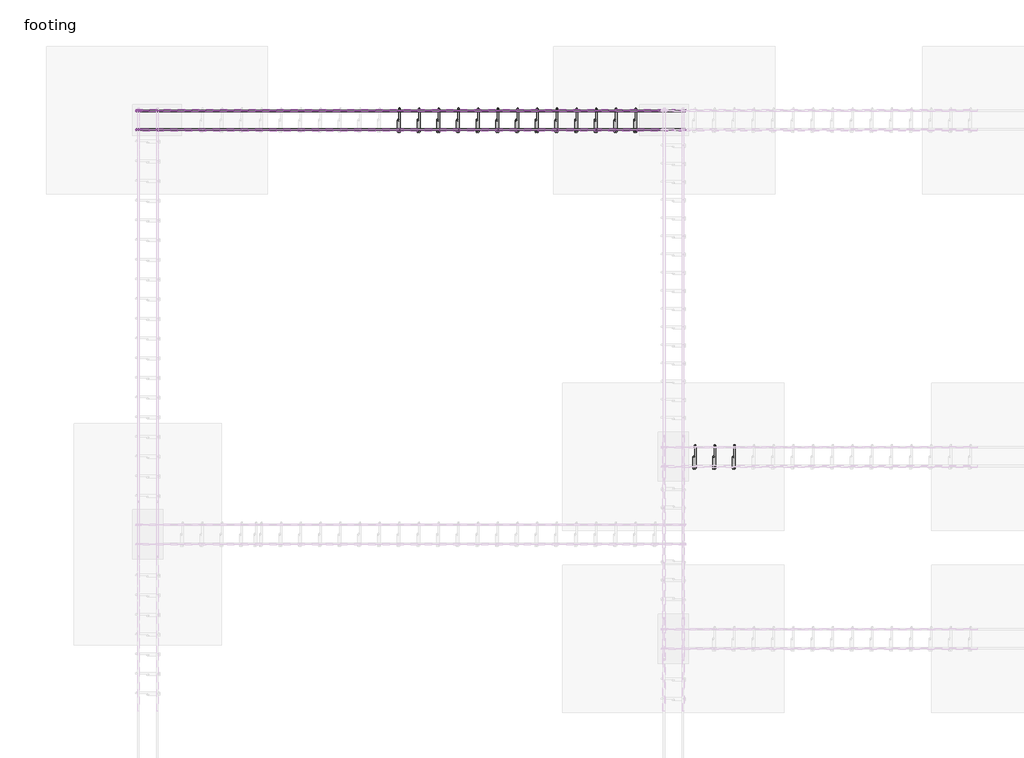
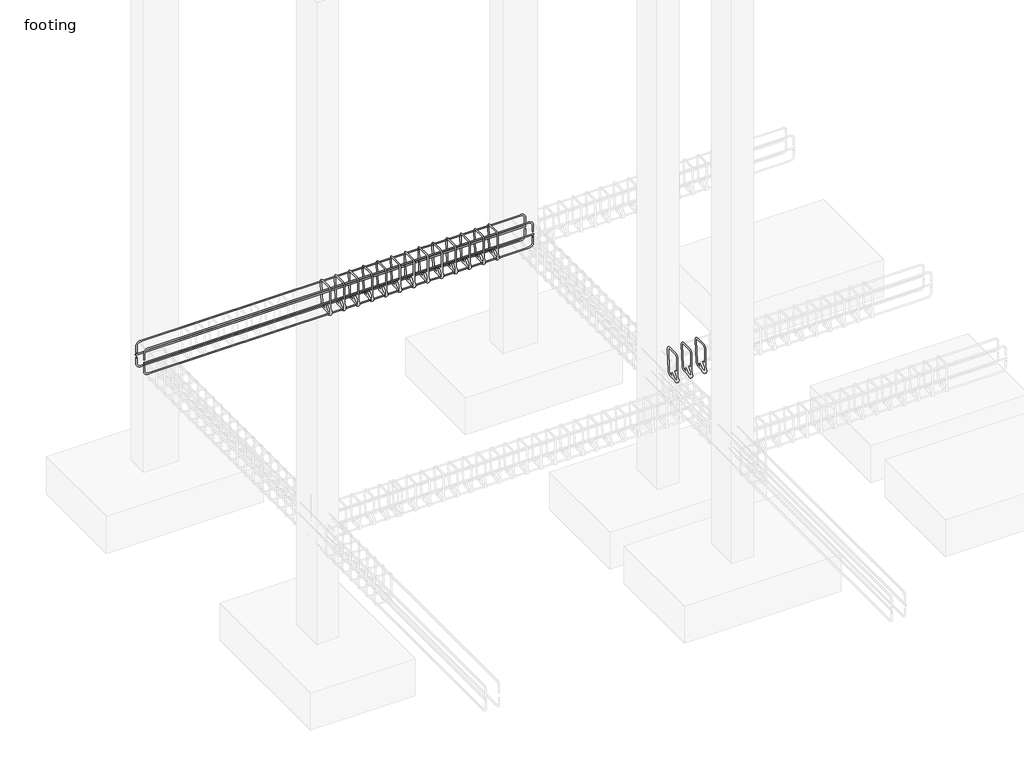
# One storey, part 17 of 21: 22 reinforcing bars.
"""IFC4 building model written with IfcOpenShell, lengths in millimetres."""

from ifc_helpers import new_model, si_unit, point, frame, origin, place, context, project, spatial, polyline, circle_curve, trimmed, segment, composite_curve, element, save
from ifc_brep_helpers import swept_disk

model = new_model("IFC4")

# Units and contexts
model_context = context("Model", 3, world=origin())
ifc_project = project(units=[si_unit("LENGTHUNIT", "METRE", prefix="MILLI")], contexts=[model_context])

# Site, building, storey
site = spatial("IfcSite", under=ifc_project)
building = spatial("IfcBuilding", under=site)
storey = spatial("IfcBuildingStorey", under=building, Name="footing", Elevation=-1524.0)

# Reinforcing bars
placement = place(None, origin())
element("IfcReinforcingBar", 1, at=placement, inside=storey, context=model_context, shape_type="SolidModel", body=[
    swept_disk(composite_curve([segment(polyline([(-7699.7883428, 8213.6387132, -310.8825168), (-7699.7883428, 8158.7737147, -365.7475153)]), True, "CONTINUOUS"), segment(trimmed(circle_curve(frame((-7699.7883428, 8136.3230744, -343.296875), z_axis=(-1.0, 0.0, 0.0), x_axis=(0.0, 22.450640299999577, -22.450640299999975)), 31.75), [point((-7699.7883428, 8158.7737147, -365.7475153))], [point((-7699.7883428, 8104.5730744, -343.296875))], True, "CARTESIAN"), True, "CONTINUOUS"), segment(polyline([(-7699.7883428, 8104.5730744, -343.296875), (-7699.7883428, 8104.5730744, -63.103125)]), True, "CONTINUOUS"), segment(trimmed(circle_curve(frame((-7699.7883428, 8136.3230744, -63.103125), z_axis=(-1.0, 0.0, 0.0), x_axis=(0.0, -31.75, 0.0)), 31.75), [point((-7699.7883428, 8104.5730744, -63.103125))], [point((-7699.7883428, 8136.3230744, -31.353125))], True, "CARTESIAN"), True, "CONTINUOUS"), segment(polyline([(-7699.7883428, 8136.3230744, -31.353125), (-7699.7883428, 8264.1168244, -31.353125)]), True, "CONTINUOUS"), segment(trimmed(circle_curve(frame((-7698.6159328, 8264.1168244, -63.0814712), z_axis=(-0.9993179916193466, 0.0, -0.03692629992126919), x_axis=(-1.1724099999992177, 0.0, 31.728346200000004)), 31.75), [point((-7699.7883428, 8264.1168244, -31.353125))], [point((-7698.6159328, 8295.8668244, -63.0814712))], True, "CARTESIAN"), True, "CONTINUOUS"), segment(polyline([(-7698.6159328, 8295.8668244, -63.0814712), (-7688.2607528, 8295.8668244, -343.3185288)]), True, "CONTINUOUS"), segment(trimmed(circle_curve(frame((-7688.2607528, 8264.1168244, -343.3185288), z_axis=(-0.9993179916193466, 0.0, -0.03692629992126919), x_axis=(0.0, 31.75, 0.0)), 31.75), [point((-7688.2607528, 8295.8668244, -343.3185288))], [point((-7687.0883428, 8264.1168244, -375.046875))], True, "CARTESIAN"), True, "CONTINUOUS"), segment(polyline([(-7687.0883428, 8264.1168244, -375.046875), (-7687.0883428, 8136.3230744, -375.046875)]), True, "CONTINUOUS"), segment(trimmed(circle_curve(frame((-7687.0883428, 8136.3230744, -343.296875), z_axis=(-1.0, 0.0, 0.0), x_axis=(0.0, 0.0, -31.75)), 31.75), [point((-7687.0883428, 8136.3230744, -375.046875))], [point((-7687.0883428, 8113.8724341, -320.8462347))], True, "CARTESIAN"), True, "CONTINUOUS"), segment(polyline([(-7687.0883428, 8113.8724341, -320.8462347), (-7687.0883428, 8168.7374326, -265.9812362)]), True, "CONTINUOUS")], self_intersect=False), 6.35),
])
element("IfcReinforcingBar", 2, at=placement, inside=storey, context=model_context, shape_type="SolidModel", body=[
    swept_disk(composite_curve([segment(polyline([(-7537.0883428, 8213.6387132, -310.8825168), (-7537.0883428, 8158.7737147, -365.7475153)]), True, "CONTINUOUS"), segment(trimmed(circle_curve(frame((-7537.0883428, 8136.3230744, -343.296875), z_axis=(-1.0, 0.0, 0.0), x_axis=(0.0, 22.450640299999577, -22.450640299999975)), 31.75), [point((-7537.0883428, 8158.7737147, -365.7475153))], [point((-7537.0883428, 8104.5730744, -343.296875))], True, "CARTESIAN"), True, "CONTINUOUS"), segment(polyline([(-7537.0883428, 8104.5730744, -343.296875), (-7537.0883428, 8104.5730744, -63.103125)]), True, "CONTINUOUS"), segment(trimmed(circle_curve(frame((-7537.0883428, 8136.3230744, -63.103125), z_axis=(-1.0, 0.0, 0.0), x_axis=(0.0, -31.75, 0.0)), 31.75), [point((-7537.0883428, 8104.5730744, -63.103125))], [point((-7537.0883428, 8136.3230744, -31.353125))], True, "CARTESIAN"), True, "CONTINUOUS"), segment(polyline([(-7537.0883428, 8136.3230744, -31.353125), (-7537.0883428, 8264.1168244, -31.353125)]), True, "CONTINUOUS"), segment(trimmed(circle_curve(frame((-7535.9159328, 8264.1168244, -63.0814712), z_axis=(-0.9993179916193466, 0.0, -0.03692629992126919), x_axis=(-1.1724100000001272, 0.0, 31.728346200000004)), 31.75), [point((-7537.0883428, 8264.1168244, -31.353125))], [point((-7535.9159328, 8295.8668244, -63.0814712))], True, "CARTESIAN"), True, "CONTINUOUS"), segment(polyline([(-7535.9159328, 8295.8668244, -63.0814712), (-7525.5607528, 8295.8668244, -343.3185288)]), True, "CONTINUOUS"), segment(trimmed(circle_curve(frame((-7525.5607528, 8264.1168244, -343.3185288), z_axis=(-0.9993179916193466, 0.0, -0.03692629992126919), x_axis=(0.0, 31.75, 0.0)), 31.75), [point((-7525.5607528, 8295.8668244, -343.3185288))], [point((-7524.3883428, 8264.1168244, -375.046875))], True, "CARTESIAN"), True, "CONTINUOUS"), segment(polyline([(-7524.3883428, 8264.1168244, -375.046875), (-7524.3883428, 8136.3230744, -375.046875)]), True, "CONTINUOUS"), segment(trimmed(circle_curve(frame((-7524.3883428, 8136.3230744, -343.296875), z_axis=(-1.0, 0.0, 0.0), x_axis=(0.0, 0.0, -31.75)), 31.75), [point((-7524.3883428, 8136.3230744, -375.046875))], [point((-7524.3883428, 8113.8724341, -320.8462347))], True, "CARTESIAN"), True, "CONTINUOUS"), segment(polyline([(-7524.3883428, 8113.8724341, -320.8462347), (-7524.3883428, 8168.7374326, -265.9812362)]), True, "CONTINUOUS")], self_intersect=False), 6.35),
])
element("IfcReinforcingBar", 3, at=placement, inside=storey, context=model_context, shape_type="SolidModel", body=[
    swept_disk(composite_curve([segment(polyline([(-7374.3883428, 8213.6387132, -310.8825168), (-7374.3883428, 8158.7737147, -365.7475153)]), True, "CONTINUOUS"), segment(trimmed(circle_curve(frame((-7374.3883428, 8136.3230744, -343.296875), z_axis=(-1.0, 0.0, 0.0), x_axis=(0.0, 22.450640299999577, -22.450640299999975)), 31.75), [point((-7374.3883428, 8158.7737147, -365.7475153))], [point((-7374.3883428, 8104.5730744, -343.296875))], True, "CARTESIAN"), True, "CONTINUOUS"), segment(polyline([(-7374.3883428, 8104.5730744, -343.296875), (-7374.3883428, 8104.5730744, -63.103125)]), True, "CONTINUOUS"), segment(trimmed(circle_curve(frame((-7374.3883428, 8136.3230744, -63.103125), z_axis=(-1.0, 0.0, 0.0), x_axis=(0.0, -31.75, 0.0)), 31.75), [point((-7374.3883428, 8104.5730744, -63.103125))], [point((-7374.3883428, 8136.3230744, -31.353125))], True, "CARTESIAN"), True, "CONTINUOUS"), segment(polyline([(-7374.3883428, 8136.3230744, -31.353125), (-7374.3883428, 8264.1168244, -31.353125)]), True, "CONTINUOUS"), segment(trimmed(circle_curve(frame((-7373.2159328, 8264.1168244, -63.0814712), z_axis=(-0.9993179916193466, 0.0, -0.03692629992126919), x_axis=(-1.1724100000001272, 0.0, 31.728346200000004)), 31.75), [point((-7374.3883428, 8264.1168244, -31.353125))], [point((-7373.2159328, 8295.8668244, -63.0814712))], True, "CARTESIAN"), True, "CONTINUOUS"), segment(polyline([(-7373.2159328, 8295.8668244, -63.0814712), (-7362.8607528, 8295.8668244, -343.3185288)]), True, "CONTINUOUS"), segment(trimmed(circle_curve(frame((-7362.8607528, 8264.1168244, -343.3185288), z_axis=(-0.9993179916193466, 0.0, -0.03692629992126919), x_axis=(0.0, 31.75, 0.0)), 31.75), [point((-7362.8607528, 8295.8668244, -343.3185288))], [point((-7361.6883428, 8264.1168244, -375.046875))], True, "CARTESIAN"), True, "CONTINUOUS"), segment(polyline([(-7361.6883428, 8264.1168244, -375.046875), (-7361.6883428, 8136.3230744, -375.046875)]), True, "CONTINUOUS"), segment(trimmed(circle_curve(frame((-7361.6883428, 8136.3230744, -343.296875), z_axis=(-1.0, 0.0, 0.0), x_axis=(0.0, 0.0, -31.75)), 31.75), [point((-7361.6883428, 8136.3230744, -375.046875))], [point((-7361.6883428, 8113.8724341, -320.8462347))], True, "CARTESIAN"), True, "CONTINUOUS"), segment(polyline([(-7361.6883428, 8113.8724341, -320.8462347), (-7361.6883428, 8168.7374326, -265.9812362)]), True, "CONTINUOUS")], self_intersect=False), 6.35),
])
element("IfcReinforcingBar", 4, at=placement, inside=storey, context=model_context, shape_type="SolidModel", body=[
    swept_disk(composite_curve([segment(polyline([(-10142.5883428, 10994.9387132, -310.8825168), (-10142.5883428, 10940.0737147, -365.7475153)]), True, "CONTINUOUS"), segment(trimmed(circle_curve(frame((-10142.5883428, 10917.6230744, -343.296875), z_axis=(-1.0, 0.0, 0.0), x_axis=(0.0, 22.450640299999577, -22.450640299999975)), 31.75), [point((-10142.5883428, 10940.0737147, -365.7475153))], [point((-10142.5883428, 10885.8730744, -343.296875))], True, "CARTESIAN"), True, "CONTINUOUS"), segment(polyline([(-10142.5883428, 10885.8730744, -343.296875), (-10142.5883428, 10885.8730744, -63.103125)]), True, "CONTINUOUS"), segment(trimmed(circle_curve(frame((-10142.5883428, 10917.6230744, -63.103125), z_axis=(-1.0, 0.0, 0.0), x_axis=(0.0, -31.75, 0.0)), 31.75), [point((-10142.5883428, 10885.8730744, -63.103125))], [point((-10142.5883428, 10917.6230744, -31.353125))], True, "CARTESIAN"), True, "CONTINUOUS"), segment(polyline([(-10142.5883428, 10917.6230744, -31.353125), (-10142.5883428, 11045.4168244, -31.353125)]), True, "CONTINUOUS"), segment(trimmed(circle_curve(frame((-10141.4159328, 11045.4168244, -63.0814712), z_axis=(-0.9993179916193466, 0.0, -0.03692629992126919), x_axis=(-1.1724099999992177, 0.0, 31.728346200000004)), 31.75), [point((-10142.5883428, 11045.4168244, -31.353125))], [point((-10141.4159328, 11077.1668244, -63.0814712))], True, "CARTESIAN"), True, "CONTINUOUS"), segment(polyline([(-10141.4159328, 11077.1668244, -63.0814712), (-10131.0607528, 11077.1668244, -343.3185288)]), True, "CONTINUOUS"), segment(trimmed(circle_curve(frame((-10131.0607528, 11045.4168244, -343.3185288), z_axis=(-0.9993179916193466, 0.0, -0.03692629992126919), x_axis=(0.0, 31.75, 0.0)), 31.75), [point((-10131.0607528, 11077.1668244, -343.3185288))], [point((-10129.8883428, 11045.4168244, -375.046875))], True, "CARTESIAN"), True, "CONTINUOUS"), segment(polyline([(-10129.8883428, 11045.4168244, -375.046875), (-10129.8883428, 10917.6230744, -375.046875)]), True, "CONTINUOUS"), segment(trimmed(circle_curve(frame((-10129.8883428, 10917.6230744, -343.296875), z_axis=(-1.0, 0.0, 0.0), x_axis=(0.0, 0.0, -31.75)), 31.75), [point((-10129.8883428, 10917.6230744, -375.046875))], [point((-10129.8883428, 10895.1724341, -320.8462347))], True, "CARTESIAN"), True, "CONTINUOUS"), segment(polyline([(-10129.8883428, 10895.1724341, -320.8462347), (-10129.8883428, 10950.0374326, -265.9812362)]), True, "CONTINUOUS")], self_intersect=False), 6.35),
])
element("IfcReinforcingBar", 5, at=placement, inside=storey, context=model_context, shape_type="SolidModel", body=[
    swept_disk(composite_curve([segment(polyline([(-9979.8883428, 10994.9387132, -310.8825168), (-9979.8883428, 10940.0737147, -365.7475153)]), True, "CONTINUOUS"), segment(trimmed(circle_curve(frame((-9979.8883428, 10917.6230744, -343.296875), z_axis=(-1.0, 0.0, 0.0), x_axis=(0.0, 22.450640299999577, -22.450640299999975)), 31.75), [point((-9979.8883428, 10940.0737147, -365.7475153))], [point((-9979.8883428, 10885.8730744, -343.296875))], True, "CARTESIAN"), True, "CONTINUOUS"), segment(polyline([(-9979.8883428, 10885.8730744, -343.296875), (-9979.8883428, 10885.8730744, -63.103125)]), True, "CONTINUOUS"), segment(trimmed(circle_curve(frame((-9979.8883428, 10917.6230744, -63.103125), z_axis=(-1.0, 0.0, 0.0), x_axis=(0.0, -31.75, 0.0)), 31.75), [point((-9979.8883428, 10885.8730744, -63.103125))], [point((-9979.8883428, 10917.6230744, -31.353125))], True, "CARTESIAN"), True, "CONTINUOUS"), segment(polyline([(-9979.8883428, 10917.6230744, -31.353125), (-9979.8883428, 11045.4168244, -31.353125)]), True, "CONTINUOUS"), segment(trimmed(circle_curve(frame((-9978.7159328, 11045.4168244, -63.0814712), z_axis=(-0.9993179916193466, 0.0, -0.03692629992126919), x_axis=(-1.1724100000010367, 0.0, 31.728346200000004)), 31.75), [point((-9979.8883428, 11045.4168244, -31.353125))], [point((-9978.7159328, 11077.1668244, -63.0814712))], True, "CARTESIAN"), True, "CONTINUOUS"), segment(polyline([(-9978.7159328, 11077.1668244, -63.0814712), (-9968.3607528, 11077.1668244, -343.3185288)]), True, "CONTINUOUS"), segment(trimmed(circle_curve(frame((-9968.3607528, 11045.4168244, -343.3185288), z_axis=(-0.9993179916193466, 0.0, -0.03692629992126919), x_axis=(0.0, 31.75, 0.0)), 31.75), [point((-9968.3607528, 11077.1668244, -343.3185288))], [point((-9967.1883428, 11045.4168244, -375.046875))], True, "CARTESIAN"), True, "CONTINUOUS"), segment(polyline([(-9967.1883428, 11045.4168244, -375.046875), (-9967.1883428, 10917.6230744, -375.046875)]), True, "CONTINUOUS"), segment(trimmed(circle_curve(frame((-9967.1883428, 10917.6230744, -343.296875), z_axis=(-1.0, 0.0, 0.0), x_axis=(0.0, 0.0, -31.75)), 31.75), [point((-9967.1883428, 10917.6230744, -375.046875))], [point((-9967.1883428, 10895.1724341, -320.8462347))], True, "CARTESIAN"), True, "CONTINUOUS"), segment(polyline([(-9967.1883428, 10895.1724341, -320.8462347), (-9967.1883428, 10950.0374326, -265.9812362)]), True, "CONTINUOUS")], self_intersect=False), 6.35),
])
element("IfcReinforcingBar", 6, at=placement, inside=storey, context=model_context, shape_type="SolidModel", body=[
    swept_disk(composite_curve([segment(polyline([(-9817.1883428, 10994.9387132, -310.8825168), (-9817.1883428, 10940.0737147, -365.7475153)]), True, "CONTINUOUS"), segment(trimmed(circle_curve(frame((-9817.1883428, 10917.6230744, -343.296875), z_axis=(-1.0, 0.0, 0.0), x_axis=(0.0, 22.450640299999577, -22.450640299999975)), 31.75), [point((-9817.1883428, 10940.0737147, -365.7475153))], [point((-9817.1883428, 10885.8730744, -343.296875))], True, "CARTESIAN"), True, "CONTINUOUS"), segment(polyline([(-9817.1883428, 10885.8730744, -343.296875), (-9817.1883428, 10885.8730744, -63.103125)]), True, "CONTINUOUS"), segment(trimmed(circle_curve(frame((-9817.1883428, 10917.6230744, -63.103125), z_axis=(-1.0, 0.0, 0.0), x_axis=(0.0, -31.75, 0.0)), 31.75), [point((-9817.1883428, 10885.8730744, -63.103125))], [point((-9817.1883428, 10917.6230744, -31.353125))], True, "CARTESIAN"), True, "CONTINUOUS"), segment(polyline([(-9817.1883428, 10917.6230744, -31.353125), (-9817.1883428, 11045.4168244, -31.353125)]), True, "CONTINUOUS"), segment(trimmed(circle_curve(frame((-9816.0159328, 11045.4168244, -63.0814712), z_axis=(-0.9993179916193466, 0.0, -0.03692629992126919), x_axis=(-1.1724099999992177, 0.0, 31.728346200000004)), 31.75), [point((-9817.1883428, 11045.4168244, -31.353125))], [point((-9816.0159328, 11077.1668244, -63.0814712))], True, "CARTESIAN"), True, "CONTINUOUS"), segment(polyline([(-9816.0159328, 11077.1668244, -63.0814712), (-9805.6607528, 11077.1668244, -343.3185288)]), True, "CONTINUOUS"), segment(trimmed(circle_curve(frame((-9805.6607528, 11045.4168244, -343.3185288), z_axis=(-0.9993179916193466, 0.0, -0.03692629992126919), x_axis=(0.0, 31.75, 0.0)), 31.75), [point((-9805.6607528, 11077.1668244, -343.3185288))], [point((-9804.4883428, 11045.4168244, -375.046875))], True, "CARTESIAN"), True, "CONTINUOUS"), segment(polyline([(-9804.4883428, 11045.4168244, -375.046875), (-9804.4883428, 10917.6230744, -375.046875)]), True, "CONTINUOUS"), segment(trimmed(circle_curve(frame((-9804.4883428, 10917.6230744, -343.296875), z_axis=(-1.0, 0.0, 0.0), x_axis=(0.0, 0.0, -31.75)), 31.75), [point((-9804.4883428, 10917.6230744, -375.046875))], [point((-9804.4883428, 10895.1724341, -320.8462347))], True, "CARTESIAN"), True, "CONTINUOUS"), segment(polyline([(-9804.4883428, 10895.1724341, -320.8462347), (-9804.4883428, 10950.0374326, -265.9812362)]), True, "CONTINUOUS")], self_intersect=False), 6.35),
])
element("IfcReinforcingBar", 7, at=placement, inside=storey, context=model_context, shape_type="SolidModel", body=[
    swept_disk(composite_curve([segment(polyline([(-9654.4883428, 10994.9387132, -310.8825168), (-9654.4883428, 10940.0737147, -365.7475153)]), True, "CONTINUOUS"), segment(trimmed(circle_curve(frame((-9654.4883428, 10917.6230744, -343.296875), z_axis=(-1.0, 0.0, 0.0), x_axis=(0.0, 22.450640299999577, -22.450640299999975)), 31.75), [point((-9654.4883428, 10940.0737147, -365.7475153))], [point((-9654.4883428, 10885.8730744, -343.296875))], True, "CARTESIAN"), True, "CONTINUOUS"), segment(polyline([(-9654.4883428, 10885.8730744, -343.296875), (-9654.4883428, 10885.8730744, -63.103125)]), True, "CONTINUOUS"), segment(trimmed(circle_curve(frame((-9654.4883428, 10917.6230744, -63.103125), z_axis=(-1.0, 0.0, 0.0), x_axis=(0.0, -31.75, 0.0)), 31.75), [point((-9654.4883428, 10885.8730744, -63.103125))], [point((-9654.4883428, 10917.6230744, -31.353125))], True, "CARTESIAN"), True, "CONTINUOUS"), segment(polyline([(-9654.4883428, 10917.6230744, -31.353125), (-9654.4883428, 11045.4168244, -31.353125)]), True, "CONTINUOUS"), segment(trimmed(circle_curve(frame((-9653.3159328, 11045.4168244, -63.0814712), z_axis=(-0.9993179916193466, 0.0, -0.03692629992126919), x_axis=(-1.1724099999992177, 0.0, 31.728346200000004)), 31.75), [point((-9654.4883428, 11045.4168244, -31.353125))], [point((-9653.3159328, 11077.1668244, -63.0814712))], True, "CARTESIAN"), True, "CONTINUOUS"), segment(polyline([(-9653.3159328, 11077.1668244, -63.0814712), (-9642.9607528, 11077.1668244, -343.3185288)]), True, "CONTINUOUS"), segment(trimmed(circle_curve(frame((-9642.9607528, 11045.4168244, -343.3185288), z_axis=(-0.9993179916193466, 0.0, -0.03692629992126919), x_axis=(0.0, 31.75, 0.0)), 31.75), [point((-9642.9607528, 11077.1668244, -343.3185288))], [point((-9641.7883428, 11045.4168244, -375.046875))], True, "CARTESIAN"), True, "CONTINUOUS"), segment(polyline([(-9641.7883428, 11045.4168244, -375.046875), (-9641.7883428, 10917.6230744, -375.046875)]), True, "CONTINUOUS"), segment(trimmed(circle_curve(frame((-9641.7883428, 10917.6230744, -343.296875), z_axis=(-1.0, 0.0, 0.0), x_axis=(0.0, 0.0, -31.75)), 31.75), [point((-9641.7883428, 10917.6230744, -375.046875))], [point((-9641.7883428, 10895.1724341, -320.8462347))], True, "CARTESIAN"), True, "CONTINUOUS"), segment(polyline([(-9641.7883428, 10895.1724341, -320.8462347), (-9641.7883428, 10950.0374326, -265.9812362)]), True, "CONTINUOUS")], self_intersect=False), 6.35),
])
element("IfcReinforcingBar", 8, at=placement, inside=storey, context=model_context, shape_type="SolidModel", body=[
    swept_disk(composite_curve([segment(polyline([(-9491.7883428, 10994.9387132, -310.8825168), (-9491.7883428, 10940.0737147, -365.7475153)]), True, "CONTINUOUS"), segment(trimmed(circle_curve(frame((-9491.7883428, 10917.6230744, -343.296875), z_axis=(-1.0, 0.0, 0.0), x_axis=(0.0, 22.450640299999577, -22.450640299999975)), 31.75), [point((-9491.7883428, 10940.0737147, -365.7475153))], [point((-9491.7883428, 10885.8730744, -343.296875))], True, "CARTESIAN"), True, "CONTINUOUS"), segment(polyline([(-9491.7883428, 10885.8730744, -343.296875), (-9491.7883428, 10885.8730744, -63.103125)]), True, "CONTINUOUS"), segment(trimmed(circle_curve(frame((-9491.7883428, 10917.6230744, -63.103125), z_axis=(-1.0, 0.0, 0.0), x_axis=(0.0, -31.75, 0.0)), 31.75), [point((-9491.7883428, 10885.8730744, -63.103125))], [point((-9491.7883428, 10917.6230744, -31.353125))], True, "CARTESIAN"), True, "CONTINUOUS"), segment(polyline([(-9491.7883428, 10917.6230744, -31.353125), (-9491.7883428, 11045.4168244, -31.353125)]), True, "CONTINUOUS"), segment(trimmed(circle_curve(frame((-9490.6159328, 11045.4168244, -63.0814712), z_axis=(-0.9993179916193466, 0.0, -0.03692629992126919), x_axis=(-1.1724100000010367, 0.0, 31.728346200000004)), 31.75), [point((-9491.7883428, 11045.4168244, -31.353125))], [point((-9490.6159328, 11077.1668244, -63.0814712))], True, "CARTESIAN"), True, "CONTINUOUS"), segment(polyline([(-9490.6159328, 11077.1668244, -63.0814712), (-9480.2607528, 11077.1668244, -343.3185288)]), True, "CONTINUOUS"), segment(trimmed(circle_curve(frame((-9480.2607528, 11045.4168244, -343.3185288), z_axis=(-0.9993179916193466, 0.0, -0.03692629992126919), x_axis=(0.0, 31.75, 0.0)), 31.75), [point((-9480.2607528, 11077.1668244, -343.3185288))], [point((-9479.0883428, 11045.4168244, -375.046875))], True, "CARTESIAN"), True, "CONTINUOUS"), segment(polyline([(-9479.0883428, 11045.4168244, -375.046875), (-9479.0883428, 10917.6230744, -375.046875)]), True, "CONTINUOUS"), segment(trimmed(circle_curve(frame((-9479.0883428, 10917.6230744, -343.296875), z_axis=(-1.0, 0.0, 0.0), x_axis=(0.0, 0.0, -31.75)), 31.75), [point((-9479.0883428, 10917.6230744, -375.046875))], [point((-9479.0883428, 10895.1724341, -320.8462347))], True, "CARTESIAN"), True, "CONTINUOUS"), segment(polyline([(-9479.0883428, 10895.1724341, -320.8462347), (-9479.0883428, 10950.0374326, -265.9812362)]), True, "CONTINUOUS")], self_intersect=False), 6.35),
])
element("IfcReinforcingBar", 9, at=placement, inside=storey, context=model_context, shape_type="SolidModel", body=[
    swept_disk(composite_curve([segment(polyline([(-9329.0883428, 10994.9387132, -310.8825168), (-9329.0883428, 10940.0737147, -365.7475153)]), True, "CONTINUOUS"), segment(trimmed(circle_curve(frame((-9329.0883428, 10917.6230744, -343.296875), z_axis=(-1.0, 0.0, 0.0), x_axis=(0.0, 22.450640299999577, -22.450640299999975)), 31.75), [point((-9329.0883428, 10940.0737147, -365.7475153))], [point((-9329.0883428, 10885.8730744, -343.296875))], True, "CARTESIAN"), True, "CONTINUOUS"), segment(polyline([(-9329.0883428, 10885.8730744, -343.296875), (-9329.0883428, 10885.8730744, -63.103125)]), True, "CONTINUOUS"), segment(trimmed(circle_curve(frame((-9329.0883428, 10917.6230744, -63.103125), z_axis=(-1.0, 0.0, 0.0), x_axis=(0.0, -31.75, 0.0)), 31.75), [point((-9329.0883428, 10885.8730744, -63.103125))], [point((-9329.0883428, 10917.6230744, -31.353125))], True, "CARTESIAN"), True, "CONTINUOUS"), segment(polyline([(-9329.0883428, 10917.6230744, -31.353125), (-9329.0883428, 11045.4168244, -31.353125)]), True, "CONTINUOUS"), segment(trimmed(circle_curve(frame((-9327.9159328, 11045.4168244, -63.0814712), z_axis=(-0.9993179916193466, 0.0, -0.03692629992126919), x_axis=(-1.1724099999992177, 0.0, 31.728346200000004)), 31.75), [point((-9329.0883428, 11045.4168244, -31.353125))], [point((-9327.9159328, 11077.1668244, -63.0814712))], True, "CARTESIAN"), True, "CONTINUOUS"), segment(polyline([(-9327.9159328, 11077.1668244, -63.0814712), (-9317.5607528, 11077.1668244, -343.3185288)]), True, "CONTINUOUS"), segment(trimmed(circle_curve(frame((-9317.5607528, 11045.4168244, -343.3185288), z_axis=(-0.9993179916193466, 0.0, -0.03692629992126919), x_axis=(0.0, 31.75, 0.0)), 31.75), [point((-9317.5607528, 11077.1668244, -343.3185288))], [point((-9316.3883428, 11045.4168244, -375.046875))], True, "CARTESIAN"), True, "CONTINUOUS"), segment(polyline([(-9316.3883428, 11045.4168244, -375.046875), (-9316.3883428, 10917.6230744, -375.046875)]), True, "CONTINUOUS"), segment(trimmed(circle_curve(frame((-9316.3883428, 10917.6230744, -343.296875), z_axis=(-1.0, 0.0, 0.0), x_axis=(0.0, 0.0, -31.75)), 31.75), [point((-9316.3883428, 10917.6230744, -375.046875))], [point((-9316.3883428, 10895.1724341, -320.8462347))], True, "CARTESIAN"), True, "CONTINUOUS"), segment(polyline([(-9316.3883428, 10895.1724341, -320.8462347), (-9316.3883428, 10950.0374326, -265.9812362)]), True, "CONTINUOUS")], self_intersect=False), 6.35),
])
element("IfcReinforcingBar", 10, at=placement, inside=storey, context=model_context, shape_type="SolidModel", body=[
    swept_disk(composite_curve([segment(polyline([(-9166.3883428, 10994.9387132, -310.8825168), (-9166.3883428, 10940.0737147, -365.7475153)]), True, "CONTINUOUS"), segment(trimmed(circle_curve(frame((-9166.3883428, 10917.6230744, -343.296875), z_axis=(-1.0, 0.0, 0.0), x_axis=(0.0, 22.450640299999577, -22.450640299999975)), 31.75), [point((-9166.3883428, 10940.0737147, -365.7475153))], [point((-9166.3883428, 10885.8730744, -343.296875))], True, "CARTESIAN"), True, "CONTINUOUS"), segment(polyline([(-9166.3883428, 10885.8730744, -343.296875), (-9166.3883428, 10885.8730744, -63.103125)]), True, "CONTINUOUS"), segment(trimmed(circle_curve(frame((-9166.3883428, 10917.6230744, -63.103125), z_axis=(-1.0, 0.0, 0.0), x_axis=(0.0, -31.75, 0.0)), 31.75), [point((-9166.3883428, 10885.8730744, -63.103125))], [point((-9166.3883428, 10917.6230744, -31.353125))], True, "CARTESIAN"), True, "CONTINUOUS"), segment(polyline([(-9166.3883428, 10917.6230744, -31.353125), (-9166.3883428, 11045.4168244, -31.353125)]), True, "CONTINUOUS"), segment(trimmed(circle_curve(frame((-9165.2159328, 11045.4168244, -63.0814712), z_axis=(-0.9993179916193466, 0.0, -0.03692629992126919), x_axis=(-1.1724100000010367, 0.0, 31.728346200000004)), 31.75), [point((-9166.3883428, 11045.4168244, -31.353125))], [point((-9165.2159328, 11077.1668244, -63.0814712))], True, "CARTESIAN"), True, "CONTINUOUS"), segment(polyline([(-9165.2159328, 11077.1668244, -63.0814712), (-9154.8607528, 11077.1668244, -343.3185288)]), True, "CONTINUOUS"), segment(trimmed(circle_curve(frame((-9154.8607528, 11045.4168244, -343.3185288), z_axis=(-0.9993179916193466, 0.0, -0.03692629992126919), x_axis=(0.0, 31.75, 0.0)), 31.75), [point((-9154.8607528, 11077.1668244, -343.3185288))], [point((-9153.6883428, 11045.4168244, -375.046875))], True, "CARTESIAN"), True, "CONTINUOUS"), segment(polyline([(-9153.6883428, 11045.4168244, -375.046875), (-9153.6883428, 10917.6230744, -375.046875)]), True, "CONTINUOUS"), segment(trimmed(circle_curve(frame((-9153.6883428, 10917.6230744, -343.296875), z_axis=(-1.0, 0.0, 0.0), x_axis=(0.0, 0.0, -31.75)), 31.75), [point((-9153.6883428, 10917.6230744, -375.046875))], [point((-9153.6883428, 10895.1724341, -320.8462347))], True, "CARTESIAN"), True, "CONTINUOUS"), segment(polyline([(-9153.6883428, 10895.1724341, -320.8462347), (-9153.6883428, 10950.0374326, -265.9812362)]), True, "CONTINUOUS")], self_intersect=False), 6.35),
])
element("IfcReinforcingBar", 11, at=placement, inside=storey, context=model_context, shape_type="SolidModel", body=[
    swept_disk(composite_curve([segment(polyline([(-9003.6883428, 10994.9387132, -310.8825168), (-9003.6883428, 10940.0737147, -365.7475153)]), True, "CONTINUOUS"), segment(trimmed(circle_curve(frame((-9003.6883428, 10917.6230744, -343.296875), z_axis=(-1.0, 0.0, 0.0), x_axis=(0.0, 22.450640299999577, -22.450640299999975)), 31.75), [point((-9003.6883428, 10940.0737147, -365.7475153))], [point((-9003.6883428, 10885.8730744, -343.296875))], True, "CARTESIAN"), True, "CONTINUOUS"), segment(polyline([(-9003.6883428, 10885.8730744, -343.296875), (-9003.6883428, 10885.8730744, -63.103125)]), True, "CONTINUOUS"), segment(trimmed(circle_curve(frame((-9003.6883428, 10917.6230744, -63.103125), z_axis=(-1.0, 0.0, 0.0), x_axis=(0.0, -31.75, 0.0)), 31.75), [point((-9003.6883428, 10885.8730744, -63.103125))], [point((-9003.6883428, 10917.6230744, -31.353125))], True, "CARTESIAN"), True, "CONTINUOUS"), segment(polyline([(-9003.6883428, 10917.6230744, -31.353125), (-9003.6883428, 11045.4168244, -31.353125)]), True, "CONTINUOUS"), segment(trimmed(circle_curve(frame((-9002.5159328, 11045.4168244, -63.0814712), z_axis=(-0.9993179916193466, 0.0, -0.03692629992126919), x_axis=(-1.1724099999992177, 0.0, 31.728346200000004)), 31.75), [point((-9003.6883428, 11045.4168244, -31.353125))], [point((-9002.5159328, 11077.1668244, -63.0814712))], True, "CARTESIAN"), True, "CONTINUOUS"), segment(polyline([(-9002.5159328, 11077.1668244, -63.0814712), (-8992.1607528, 11077.1668244, -343.3185288)]), True, "CONTINUOUS"), segment(trimmed(circle_curve(frame((-8992.1607528, 11045.4168244, -343.3185288), z_axis=(-0.9993179916193466, 0.0, -0.03692629992126919), x_axis=(0.0, 31.75, 0.0)), 31.75), [point((-8992.1607528, 11077.1668244, -343.3185288))], [point((-8990.9883428, 11045.4168244, -375.046875))], True, "CARTESIAN"), True, "CONTINUOUS"), segment(polyline([(-8990.9883428, 11045.4168244, -375.046875), (-8990.9883428, 10917.6230744, -375.046875)]), True, "CONTINUOUS"), segment(trimmed(circle_curve(frame((-8990.9883428, 10917.6230744, -343.296875), z_axis=(-1.0, 0.0, 0.0), x_axis=(0.0, 0.0, -31.75)), 31.75), [point((-8990.9883428, 10917.6230744, -375.046875))], [point((-8990.9883428, 10895.1724341, -320.8462347))], True, "CARTESIAN"), True, "CONTINUOUS"), segment(polyline([(-8990.9883428, 10895.1724341, -320.8462347), (-8990.9883428, 10950.0374326, -265.9812362)]), True, "CONTINUOUS")], self_intersect=False), 6.35),
])
element("IfcReinforcingBar", 12, at=placement, inside=storey, context=model_context, shape_type="SolidModel", body=[
    swept_disk(composite_curve([segment(polyline([(-8840.9883428, 10994.9387132, -310.8825168), (-8840.9883428, 10940.0737147, -365.7475153)]), True, "CONTINUOUS"), segment(trimmed(circle_curve(frame((-8840.9883428, 10917.6230744, -343.296875), z_axis=(-1.0, 0.0, 0.0), x_axis=(0.0, 22.450640299999577, -22.450640299999975)), 31.75), [point((-8840.9883428, 10940.0737147, -365.7475153))], [point((-8840.9883428, 10885.8730744, -343.296875))], True, "CARTESIAN"), True, "CONTINUOUS"), segment(polyline([(-8840.9883428, 10885.8730744, -343.296875), (-8840.9883428, 10885.8730744, -63.103125)]), True, "CONTINUOUS"), segment(trimmed(circle_curve(frame((-8840.9883428, 10917.6230744, -63.103125), z_axis=(-1.0, 0.0, 0.0), x_axis=(0.0, -31.75, 0.0)), 31.75), [point((-8840.9883428, 10885.8730744, -63.103125))], [point((-8840.9883428, 10917.6230744, -31.353125))], True, "CARTESIAN"), True, "CONTINUOUS"), segment(polyline([(-8840.9883428, 10917.6230744, -31.353125), (-8840.9883428, 11045.4168244, -31.353125)]), True, "CONTINUOUS"), segment(trimmed(circle_curve(frame((-8839.8159328, 11045.4168244, -63.0814712), z_axis=(-0.9993179916193466, 0.0, -0.03692629992126919), x_axis=(-1.1724099999992177, 0.0, 31.728346200000004)), 31.75), [point((-8840.9883428, 11045.4168244, -31.353125))], [point((-8839.8159328, 11077.1668244, -63.0814712))], True, "CARTESIAN"), True, "CONTINUOUS"), segment(polyline([(-8839.8159328, 11077.1668244, -63.0814712), (-8829.4607528, 11077.1668244, -343.3185288)]), True, "CONTINUOUS"), segment(trimmed(circle_curve(frame((-8829.4607528, 11045.4168244, -343.3185288), z_axis=(-0.9993179916193466, 0.0, -0.03692629992126919), x_axis=(0.0, 31.75, 0.0)), 31.75), [point((-8829.4607528, 11077.1668244, -343.3185288))], [point((-8828.2883428, 11045.4168244, -375.046875))], True, "CARTESIAN"), True, "CONTINUOUS"), segment(polyline([(-8828.2883428, 11045.4168244, -375.046875), (-8828.2883428, 10917.6230744, -375.046875)]), True, "CONTINUOUS"), segment(trimmed(circle_curve(frame((-8828.2883428, 10917.6230744, -343.296875), z_axis=(-1.0, 0.0, 0.0), x_axis=(0.0, 0.0, -31.75)), 31.75), [point((-8828.2883428, 10917.6230744, -375.046875))], [point((-8828.2883428, 10895.1724341, -320.8462347))], True, "CARTESIAN"), True, "CONTINUOUS"), segment(polyline([(-8828.2883428, 10895.1724341, -320.8462347), (-8828.2883428, 10950.0374326, -265.9812362)]), True, "CONTINUOUS")], self_intersect=False), 6.35),
])
element("IfcReinforcingBar", 13, at=placement, inside=storey, context=model_context, shape_type="SolidModel", body=[
    swept_disk(composite_curve([segment(polyline([(-8678.2883428, 10994.9387132, -310.8825168), (-8678.2883428, 10940.0737147, -365.7475153)]), True, "CONTINUOUS"), segment(trimmed(circle_curve(frame((-8678.2883428, 10917.6230744, -343.296875), z_axis=(-1.0, 0.0, 0.0), x_axis=(0.0, 22.450640299999577, -22.450640299999975)), 31.75), [point((-8678.2883428, 10940.0737147, -365.7475153))], [point((-8678.2883428, 10885.8730744, -343.296875))], True, "CARTESIAN"), True, "CONTINUOUS"), segment(polyline([(-8678.2883428, 10885.8730744, -343.296875), (-8678.2883428, 10885.8730744, -63.103125)]), True, "CONTINUOUS"), segment(trimmed(circle_curve(frame((-8678.2883428, 10917.6230744, -63.103125), z_axis=(-1.0, 0.0, 0.0), x_axis=(0.0, -31.75, 0.0)), 31.75), [point((-8678.2883428, 10885.8730744, -63.103125))], [point((-8678.2883428, 10917.6230744, -31.353125))], True, "CARTESIAN"), True, "CONTINUOUS"), segment(polyline([(-8678.2883428, 10917.6230744, -31.353125), (-8678.2883428, 11045.4168244, -31.353125)]), True, "CONTINUOUS"), segment(trimmed(circle_curve(frame((-8677.1159328, 11045.4168244, -63.0814712), z_axis=(-0.9993179916193466, 0.0, -0.03692629992126919), x_axis=(-1.1724100000010367, 0.0, 31.728346200000004)), 31.75), [point((-8678.2883428, 11045.4168244, -31.353125))], [point((-8677.1159328, 11077.1668244, -63.0814712))], True, "CARTESIAN"), True, "CONTINUOUS"), segment(polyline([(-8677.1159328, 11077.1668244, -63.0814712), (-8666.7607528, 11077.1668244, -343.3185288)]), True, "CONTINUOUS"), segment(trimmed(circle_curve(frame((-8666.7607528, 11045.4168244, -343.3185288), z_axis=(-0.9993179916193466, 0.0, -0.03692629992126919), x_axis=(0.0, 31.75, 0.0)), 31.75), [point((-8666.7607528, 11077.1668244, -343.3185288))], [point((-8665.5883428, 11045.4168244, -375.046875))], True, "CARTESIAN"), True, "CONTINUOUS"), segment(polyline([(-8665.5883428, 11045.4168244, -375.046875), (-8665.5883428, 10917.6230744, -375.046875)]), True, "CONTINUOUS"), segment(trimmed(circle_curve(frame((-8665.5883428, 10917.6230744, -343.296875), z_axis=(-1.0, 0.0, 0.0), x_axis=(0.0, 0.0, -31.75)), 31.75), [point((-8665.5883428, 10917.6230744, -375.046875))], [point((-8665.5883428, 10895.1724341, -320.8462347))], True, "CARTESIAN"), True, "CONTINUOUS"), segment(polyline([(-8665.5883428, 10895.1724341, -320.8462347), (-8665.5883428, 10950.0374326, -265.9812362)]), True, "CONTINUOUS")], self_intersect=False), 6.35),
])
element("IfcReinforcingBar", 14, at=placement, inside=storey, context=model_context, shape_type="SolidModel", body=[
    swept_disk(composite_curve([segment(polyline([(-8515.5883428, 10994.9387132, -310.8825168), (-8515.5883428, 10940.0737147, -365.7475153)]), True, "CONTINUOUS"), segment(trimmed(circle_curve(frame((-8515.5883428, 10917.6230744, -343.296875), z_axis=(-1.0, 0.0, 0.0), x_axis=(0.0, 22.450640299999577, -22.450640299999975)), 31.75), [point((-8515.5883428, 10940.0737147, -365.7475153))], [point((-8515.5883428, 10885.8730744, -343.296875))], True, "CARTESIAN"), True, "CONTINUOUS"), segment(polyline([(-8515.5883428, 10885.8730744, -343.296875), (-8515.5883428, 10885.8730744, -63.103125)]), True, "CONTINUOUS"), segment(trimmed(circle_curve(frame((-8515.5883428, 10917.6230744, -63.103125), z_axis=(-1.0, 0.0, 0.0), x_axis=(0.0, -31.75, 0.0)), 31.75), [point((-8515.5883428, 10885.8730744, -63.103125))], [point((-8515.5883428, 10917.6230744, -31.353125))], True, "CARTESIAN"), True, "CONTINUOUS"), segment(polyline([(-8515.5883428, 10917.6230744, -31.353125), (-8515.5883428, 11045.4168244, -31.353125)]), True, "CONTINUOUS"), segment(trimmed(circle_curve(frame((-8514.4159328, 11045.4168244, -63.0814712), z_axis=(-0.9993179916193466, 0.0, -0.03692629992126919), x_axis=(-1.1724099999992177, 0.0, 31.728346200000004)), 31.75), [point((-8515.5883428, 11045.4168244, -31.353125))], [point((-8514.4159328, 11077.1668244, -63.0814712))], True, "CARTESIAN"), True, "CONTINUOUS"), segment(polyline([(-8514.4159328, 11077.1668244, -63.0814712), (-8504.0607528, 11077.1668244, -343.3185288)]), True, "CONTINUOUS"), segment(trimmed(circle_curve(frame((-8504.0607528, 11045.4168244, -343.3185288), z_axis=(-0.9993179916193466, 0.0, -0.03692629992126919), x_axis=(0.0, 31.75, 0.0)), 31.75), [point((-8504.0607528, 11077.1668244, -343.3185288))], [point((-8502.8883428, 11045.4168244, -375.046875))], True, "CARTESIAN"), True, "CONTINUOUS"), segment(polyline([(-8502.8883428, 11045.4168244, -375.046875), (-8502.8883428, 10917.6230744, -375.046875)]), True, "CONTINUOUS"), segment(trimmed(circle_curve(frame((-8502.8883428, 10917.6230744, -343.296875), z_axis=(-1.0, 0.0, 0.0), x_axis=(0.0, 0.0, -31.75)), 31.75), [point((-8502.8883428, 10917.6230744, -375.046875))], [point((-8502.8883428, 10895.1724341, -320.8462347))], True, "CARTESIAN"), True, "CONTINUOUS"), segment(polyline([(-8502.8883428, 10895.1724341, -320.8462347), (-8502.8883428, 10950.0374326, -265.9812362)]), True, "CONTINUOUS")], self_intersect=False), 6.35),
])
element("IfcReinforcingBar", 15, at=placement, inside=storey, context=model_context, shape_type="SolidModel", body=[
    swept_disk(composite_curve([segment(polyline([(-8352.8883428, 10994.9387132, -310.8825168), (-8352.8883428, 10940.0737147, -365.7475153)]), True, "CONTINUOUS"), segment(trimmed(circle_curve(frame((-8352.8883428, 10917.6230744, -343.296875), z_axis=(-1.0, 0.0, 0.0), x_axis=(0.0, 22.450640299999577, -22.450640299999975)), 31.75), [point((-8352.8883428, 10940.0737147, -365.7475153))], [point((-8352.8883428, 10885.8730744, -343.296875))], True, "CARTESIAN"), True, "CONTINUOUS"), segment(polyline([(-8352.8883428, 10885.8730744, -343.296875), (-8352.8883428, 10885.8730744, -63.103125)]), True, "CONTINUOUS"), segment(trimmed(circle_curve(frame((-8352.8883428, 10917.6230744, -63.103125), z_axis=(-1.0, 0.0, 0.0), x_axis=(0.0, -31.75, 0.0)), 31.75), [point((-8352.8883428, 10885.8730744, -63.103125))], [point((-8352.8883428, 10917.6230744, -31.353125))], True, "CARTESIAN"), True, "CONTINUOUS"), segment(polyline([(-8352.8883428, 10917.6230744, -31.353125), (-8352.8883428, 11045.4168244, -31.353125)]), True, "CONTINUOUS"), segment(trimmed(circle_curve(frame((-8351.7159328, 11045.4168244, -63.0814712), z_axis=(-0.9993179916193466, 0.0, -0.03692629992126919), x_axis=(-1.1724100000010367, 0.0, 31.728346200000004)), 31.75), [point((-8352.8883428, 11045.4168244, -31.353125))], [point((-8351.7159328, 11077.1668244, -63.0814712))], True, "CARTESIAN"), True, "CONTINUOUS"), segment(polyline([(-8351.7159328, 11077.1668244, -63.0814712), (-8341.3607528, 11077.1668244, -343.3185288)]), True, "CONTINUOUS"), segment(trimmed(circle_curve(frame((-8341.3607528, 11045.4168244, -343.3185288), z_axis=(-0.9993179916193466, 0.0, -0.03692629992126919), x_axis=(0.0, 31.75, 0.0)), 31.75), [point((-8341.3607528, 11077.1668244, -343.3185288))], [point((-8340.1883428, 11045.4168244, -375.046875))], True, "CARTESIAN"), True, "CONTINUOUS"), segment(polyline([(-8340.1883428, 11045.4168244, -375.046875), (-8340.1883428, 10917.6230744, -375.046875)]), True, "CONTINUOUS"), segment(trimmed(circle_curve(frame((-8340.1883428, 10917.6230744, -343.296875), z_axis=(-1.0, 0.0, 0.0), x_axis=(0.0, 0.0, -31.75)), 31.75), [point((-8340.1883428, 10917.6230744, -375.046875))], [point((-8340.1883428, 10895.1724341, -320.8462347))], True, "CARTESIAN"), True, "CONTINUOUS"), segment(polyline([(-8340.1883428, 10895.1724341, -320.8462347), (-8340.1883428, 10950.0374326, -265.9812362)]), True, "CONTINUOUS")], self_intersect=False), 6.35),
])
element("IfcReinforcingBar", 16, at=placement, inside=storey, context=model_context, shape_type="SolidModel", body=[
    swept_disk(composite_curve([segment(polyline([(-8190.1883428, 10994.9387132, -310.8825168), (-8190.1883428, 10940.0737147, -365.7475153)]), True, "CONTINUOUS"), segment(trimmed(circle_curve(frame((-8190.1883428, 10917.6230744, -343.296875), z_axis=(-1.0, 0.0, 0.0), x_axis=(0.0, 22.450640299999577, -22.450640299999975)), 31.75), [point((-8190.1883428, 10940.0737147, -365.7475153))], [point((-8190.1883428, 10885.8730744, -343.296875))], True, "CARTESIAN"), True, "CONTINUOUS"), segment(polyline([(-8190.1883428, 10885.8730744, -343.296875), (-8190.1883428, 10885.8730744, -63.103125)]), True, "CONTINUOUS"), segment(trimmed(circle_curve(frame((-8190.1883428, 10917.6230744, -63.103125), z_axis=(-1.0, 0.0, 0.0), x_axis=(0.0, -31.75, 0.0)), 31.75), [point((-8190.1883428, 10885.8730744, -63.103125))], [point((-8190.1883428, 10917.6230744, -31.353125))], True, "CARTESIAN"), True, "CONTINUOUS"), segment(polyline([(-8190.1883428, 10917.6230744, -31.353125), (-8190.1883428, 11045.4168244, -31.353125)]), True, "CONTINUOUS"), segment(trimmed(circle_curve(frame((-8189.0159328, 11045.4168244, -63.0814712), z_axis=(-0.9993179916193466, 0.0, -0.03692629992126919), x_axis=(-1.1724100000001272, 0.0, 31.728346200000004)), 31.75), [point((-8190.1883428, 11045.4168244, -31.353125))], [point((-8189.0159328, 11077.1668244, -63.0814712))], True, "CARTESIAN"), True, "CONTINUOUS"), segment(polyline([(-8189.0159328, 11077.1668244, -63.0814712), (-8178.6607528, 11077.1668244, -343.3185288)]), True, "CONTINUOUS"), segment(trimmed(circle_curve(frame((-8178.6607528, 11045.4168244, -343.3185288), z_axis=(-0.9993179916193466, 0.0, -0.03692629992126919), x_axis=(0.0, 31.75, 0.0)), 31.75), [point((-8178.6607528, 11077.1668244, -343.3185288))], [point((-8177.4883428, 11045.4168244, -375.046875))], True, "CARTESIAN"), True, "CONTINUOUS"), segment(polyline([(-8177.4883428, 11045.4168244, -375.046875), (-8177.4883428, 10917.6230744, -375.046875)]), True, "CONTINUOUS"), segment(trimmed(circle_curve(frame((-8177.4883428, 10917.6230744, -343.296875), z_axis=(-1.0, 0.0, 0.0), x_axis=(0.0, 0.0, -31.75)), 31.75), [point((-8177.4883428, 10917.6230744, -375.046875))], [point((-8177.4883428, 10895.1724341, -320.8462347))], True, "CARTESIAN"), True, "CONTINUOUS"), segment(polyline([(-8177.4883428, 10895.1724341, -320.8462347), (-8177.4883428, 10950.0374326, -265.9812362)]), True, "CONTINUOUS")], self_intersect=False), 6.35),
])
element("IfcReinforcingBar", 17, at=placement, inside=storey, context=model_context, shape_type="SolidModel", body=[
    swept_disk(composite_curve([segment(polyline([(-7770.5521673, 11058.8872086, -236.1172592), (-7770.5521673, 11058.8872086, -312.3172592)]), True, "CONTINUOUS"), segment(trimmed(circle_curve(frame((-7815.0021673, 11058.8872086, -312.3172592), z_axis=(0.0, 1.0, -2.1166279873208456e-12), x_axis=(44.44999999999982, 0.0, 0.0)), 44.45), [point((-7770.5521673, 11058.8872086, -312.3172592))], [point((-7815.0021673, 11058.8872086, -356.7672592))], True, "CARTESIAN"), True, "CONTINUOUS"), segment(polyline([(-7815.0021673, 11058.8872086, -356.7672592), (-12260.7959173, 11058.8872086, -356.7672592)]), True, "CONTINUOUS"), segment(trimmed(circle_curve(frame((-12260.7959173, 11058.8872086, -312.3172592), z_axis=(0.0, 1.0, -2.1166279873208456e-12), x_axis=(0.0, 0.0, -44.44999999999999)), 44.45), [point((-12260.7959173, 11058.8872086, -356.7672592))], [point((-12305.2459173, 11058.8872086, -312.3172592))], True, "CARTESIAN"), True, "CONTINUOUS"), segment(polyline([(-12305.2459173, 11058.8872086, -312.3172592), (-12305.2459173, 11058.8872086, -236.1172592)]), True, "CONTINUOUS")], self_intersect=False), 6.35),
])
element("IfcReinforcingBar", 18, at=placement, inside=storey, context=model_context, shape_type="SolidModel", body=[
    swept_disk(composite_curve([segment(polyline([(-7770.5521673, 10904.1526902, -170.2827408), (-7770.5521673, 10904.1526902, -94.0827408)]), True, "CONTINUOUS"), segment(trimmed(circle_curve(frame((-7815.0021673, 10904.1526902, -94.0827408), z_axis=(0.0, -1.0, 0.0), x_axis=(44.44999999999982, 0.0, 0.0)), 44.45), [point((-7770.5521673, 10904.1526902, -94.0827408))], [point((-7815.0021673, 10904.1526902, -49.6327408))], True, "CARTESIAN"), True, "CONTINUOUS"), segment(polyline([(-7815.0021673, 10904.1526902, -49.6327408), (-12260.7959173, 10904.1526902, -49.6327408)]), True, "CONTINUOUS"), segment(trimmed(circle_curve(frame((-12260.7959173, 10904.1526902, -94.0827408), z_axis=(0.0, -1.0, 0.0), x_axis=(0.0, 0.0, 44.449999999999996)), 44.45), [point((-12260.7959173, 10904.1526902, -49.6327408))], [point((-12305.2459173, 10904.1526902, -94.0827408))], True, "CARTESIAN"), True, "CONTINUOUS"), segment(polyline([(-12305.2459173, 10904.1526902, -94.0827408), (-12305.2459173, 10904.1526902, -170.2827408)]), True, "CONTINUOUS")], self_intersect=False), 6.35),
])
element("IfcReinforcingBar", 19, at=placement, inside=storey, context=model_context, shape_type="SolidModel", body=[
    swept_disk(composite_curve([segment(polyline([(-7770.5521673, 10904.1526902, -236.1172592), (-7770.5521673, 10904.1526902, -312.3172592)]), True, "CONTINUOUS"), segment(trimmed(circle_curve(frame((-7815.0021673, 10904.1526902, -312.3172592), z_axis=(0.0, 1.0, 2.1166279873208456e-12), x_axis=(44.44999999999982, 0.0, 0.0)), 44.45), [point((-7770.5521673, 10904.1526902, -312.3172592))], [point((-7815.0021673, 10904.1526902, -356.7672592))], True, "CARTESIAN"), True, "CONTINUOUS"), segment(polyline([(-7815.0021673, 10904.1526902, -356.7672592), (-12260.7959173, 10904.1526902, -356.7672592)]), True, "CONTINUOUS"), segment(trimmed(circle_curve(frame((-12260.7959173, 10904.1526902, -312.3172592), z_axis=(0.0, 1.0, 2.1166279873208456e-12), x_axis=(0.0, 0.0, -44.44999999999999)), 44.45), [point((-12260.7959173, 10904.1526902, -356.7672592))], [point((-12305.2459173, 10904.1526902, -312.3172592))], True, "CARTESIAN"), True, "CONTINUOUS"), segment(polyline([(-12305.2459173, 10904.1526902, -312.3172592), (-12305.2459173, 10904.1526902, -236.1172592)]), True, "CONTINUOUS")], self_intersect=False), 6.35),
])
element("IfcReinforcingBar", 20, at=placement, inside=storey, context=model_context, shape_type="SolidModel", body=[
    swept_disk(composite_curve([segment(polyline([(-7770.5521673, 11058.8872086, -170.2827408), (-7770.5521673, 11058.8872086, -94.0827408)]), True, "CONTINUOUS"), segment(trimmed(circle_curve(frame((-7815.0021673, 11058.8872086, -94.0827408), z_axis=(0.0, -1.0, 0.0), x_axis=(44.44999999999982, 0.0, 0.0)), 44.45), [point((-7770.5521673, 11058.8872086, -94.0827408))], [point((-7815.0021673, 11058.8872086, -49.6327408))], True, "CARTESIAN"), True, "CONTINUOUS"), segment(polyline([(-7815.0021673, 11058.8872086, -49.6327408), (-12260.7959173, 11058.8872086, -49.6327408)]), True, "CONTINUOUS"), segment(trimmed(circle_curve(frame((-12260.7959173, 11058.8872086, -94.0827408), z_axis=(0.0, -1.0, 0.0), x_axis=(0.0, 0.0, 44.449999999999996)), 44.45), [point((-12260.7959173, 11058.8872086, -49.6327408))], [point((-12305.2459173, 11058.8872086, -94.0827408))], True, "CARTESIAN"), True, "CONTINUOUS"), segment(polyline([(-12305.2459173, 11058.8872086, -94.0827408), (-12305.2459173, 11058.8872086, -170.2827408)]), True, "CONTINUOUS")], self_intersect=False), 6.35),
])
element("IfcReinforcingBar", 21, at=placement, inside=storey, context=model_context, shape_type="SolidModel", body=[
    swept_disk(composite_curve([segment(polyline([(-7764.2021673, 11064.4668244, -203.2), (-12311.5959173, 11064.4668244, -203.2)]), True, "CONTINUOUS")], self_intersect=False), 6.35),
])
element("IfcReinforcingBar", 22, at=placement, inside=storey, context=model_context, shape_type="SolidModel", body=[
    swept_disk(composite_curve([segment(polyline([(-7764.2021673, 10898.5730744, -203.2), (-12311.5959173, 10898.5730744, -203.2)]), True, "CONTINUOUS")], self_intersect=False), 6.35),
])

save(model, "model.ifc")

# Revit data of these elements
# Elements 1, 2, 3, 4, 5, 6, 7, 8, 9, 10, 11, 12, 13, 14, 15, 16, 17, 18, 19, 20, 21, 22 (IfcReinforcingBar)
#   Phase Created = New Construction
